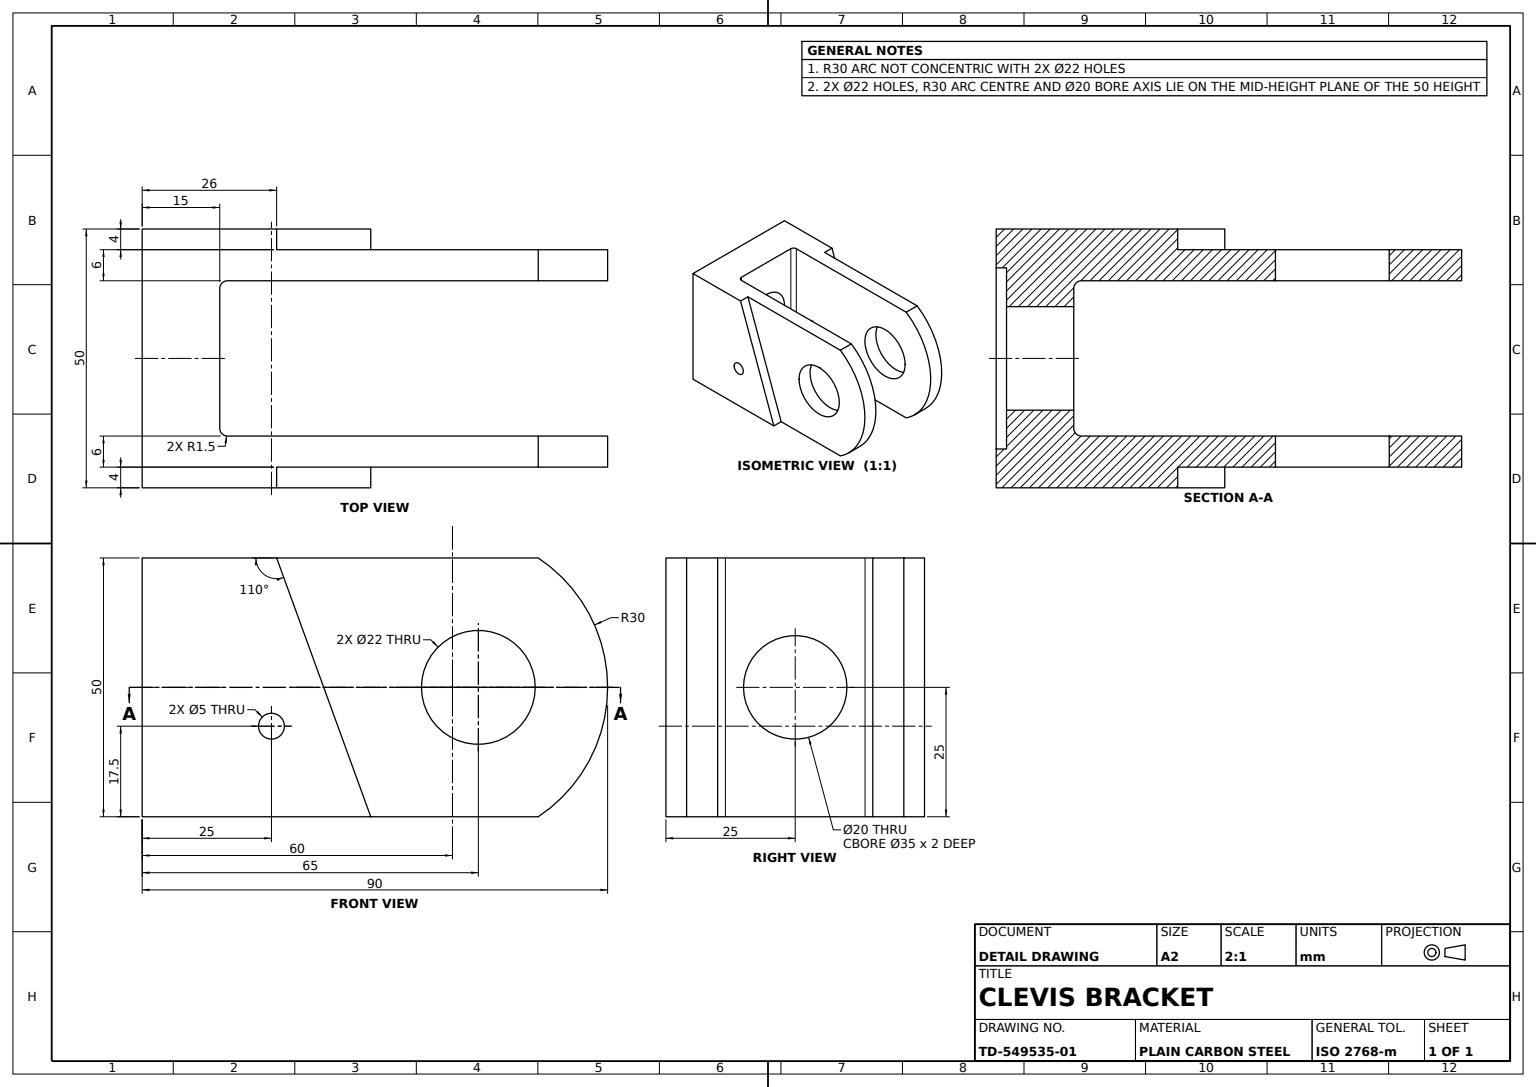
from build123d import *

# Parameters (mm, degrees)
CLEVIS_BODY_PROFILE_R   = 11
CLEVIS_BODY_PROFILE_R_2 = 2.5
CLEVIS_BODY_DEPTH       = 25
CLEVIS_SLOT_SKETCH_W    = 90.532278548
CLEVIS_SLOT_SKETCH_H    = 30
CLEVIS_SLOT_30MM_DEPTH  = 86.732140997
EAR_SIDE_RELIEF_DEPTH   = 4
SLOT_FILLET_R1_5_R      = 1.5


with BuildPart() as part:
    # Clevis Body Profile → Clevis Body (new, symmetric)
    with BuildSketch(Plane.XY):
        with BuildLine():
            Line((-65, 25), (11.583123952, 25))
            ThreePointArc((11.583123952, 25), (25, 0), (11.583123952, -25))
            Line((11.583123952, -25), (-65, -25))
            Line((-65, -25), (-65, 25))
        make_face()
        Circle(CLEVIS_BODY_PROFILE_R, mode=Mode.SUBTRACT)
        with Locations((-40, -7.5)):
            Circle(CLEVIS_BODY_PROFILE_R_2, mode=Mode.SUBTRACT)
    extrude(amount=CLEVIS_BODY_DEPTH, both=True)

    # Clevis Slot Sketch → Clevis Slot 30mm (cut, through all)
    with BuildSketch(Plane(origin=(0, 25, 0), x_dir=(1, 0, 0), z_dir=(0, 1, 0))):
        with Locations((-4.733860726, 0)):
            Rectangle(CLEVIS_SLOT_SKETCH_W, CLEVIS_SLOT_SKETCH_H)
    extrude(amount=-CLEVIS_SLOT_30MM_DEPTH, mode=Mode.SUBTRACT)

    # Ear Side Relief Sketch → Ear Side Relief (cut)
    with BuildSketch(Plane.XY.offset(25)):
        with BuildLine():
            Line((-39, 25), (-20.801488287, -25))
            Line((-20.801488287, -25), (11.583123952, -25))
            ThreePointArc((11.583123952, -25), (25, 0), (11.583123952, 25))
            Line((11.583123952, 25), (-39, 25))
        make_face()
    ear_side_relief = extrude(amount=-EAR_SIDE_RELIEF_DEPTH, mode=Mode.SUBTRACT)

    # Ear Side Relief Mirror: Ear Side Relief across plane
    add(ear_side_relief.mirror(Plane.XY), mode=Mode.SUBTRACT)

    # Slot Fillet R1.5
    slot_fillet_r1_5_edges = [part.edges().sort_by_distance(p)[0] for p in [
        (-50, 0, -15),
        (-50, 0, 15),
    ]]
    fillet(slot_fillet_r1_5_edges, radius=SLOT_FILLET_R1_5_R)

    # Sketch4 → Pin Bore Ø20 CBore Ø35 (revolve, cut)
    with BuildSketch(Plane(origin=(-65, 0, 0), x_dir=(0, 0, 1), z_dir=(0, 1, 0))):
        Polygon((0, 0), (0, 99.718353376), (10, 99.718353376), (10, 2), (17.5, 2), (17.5, 0), align=None)
    revolve(axis=Axis((45, 0, 0), (-1, 0, 0)), mode=Mode.SUBTRACT)


solid = part.part
